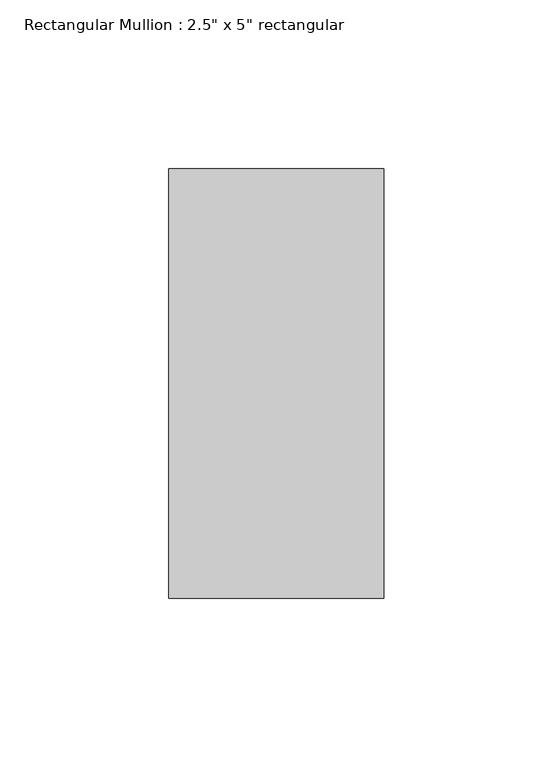
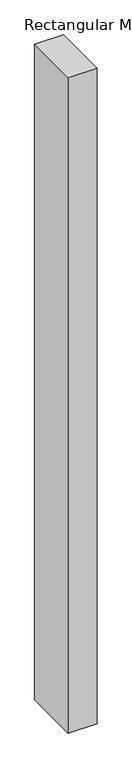
"""IFC4 building model written with IfcOpenShell, lengths in millimetres: member geometry."""

from ifc_helpers import new_model, si_unit, frame, origin, place, context, project, spatial, polyline, outline, extrude, source, transform, mapped, element, save


def member_a7b21902(model_context):
    return source(origin(), model_context, "Body", "SweptSolid", [
        extrude(outline(polyline([(31.75, 63.5), (31.75, -63.5), (-31.75, -63.5), (-31.75, 63.5), (31.75, 63.5)])), frame((0.0, 0.0, -1523.1033231), z_axis=(0.0, 0.0, 1.0), x_axis=(1.0, 0.0, 0.0)), (0.0, 0.0, 1.0), 1523.1033231),
    ])


if __name__ == "__main__":
    model = new_model("IFC4")
    model_context = context("Model", 3, world=origin())
    ifc_project = project(units=[si_unit("LENGTHUNIT", "METRE", prefix="MILLI")], contexts=[model_context])
    site = spatial("IfcSite", under=ifc_project)
    building = spatial("IfcBuilding", under=site)
    placement = place(None, origin())
    member_shape = member_a7b21902(model_context)
    element("IfcMember", 1, ObjectType="Rectangular Mullion : 2.5\" x 5\" rectangular", at=placement, inside=building, context=model_context, shape_type="MappedRepresentation", body=[
        mapped(member_shape, transform((0.0, 0.0, 0.0), x_axis=(1.0, 0.0, 0.0), y_axis=(0.0, 1.0, 0.0), z_axis=(0.0, 0.0, 1.0))),
    ])
    save(model, "model.ifc")

# Revit data of these elements
# Type "Rectangular Mullion : 2.5\" x 5\" rectangular"
#   built-in parameter 1007304 = 0.416667 (stored number, unit not read)
#   built-in parameter 1007301 = 0.104167 (stored number, unit not read)
#   built-in parameter 1007300 = 0.104167 (stored number, unit not read)
# Element 1 (IfcMember, "Rectangular Mullion : 2.5\" x 5\" rectangular")
#   Materials on its faces: "Aluminum"
# Materials
#   "Aluminum": class "Metal", colour RGB 247 247 247, transparency 0, Description = "Aluminum 6061", Cost = 0
